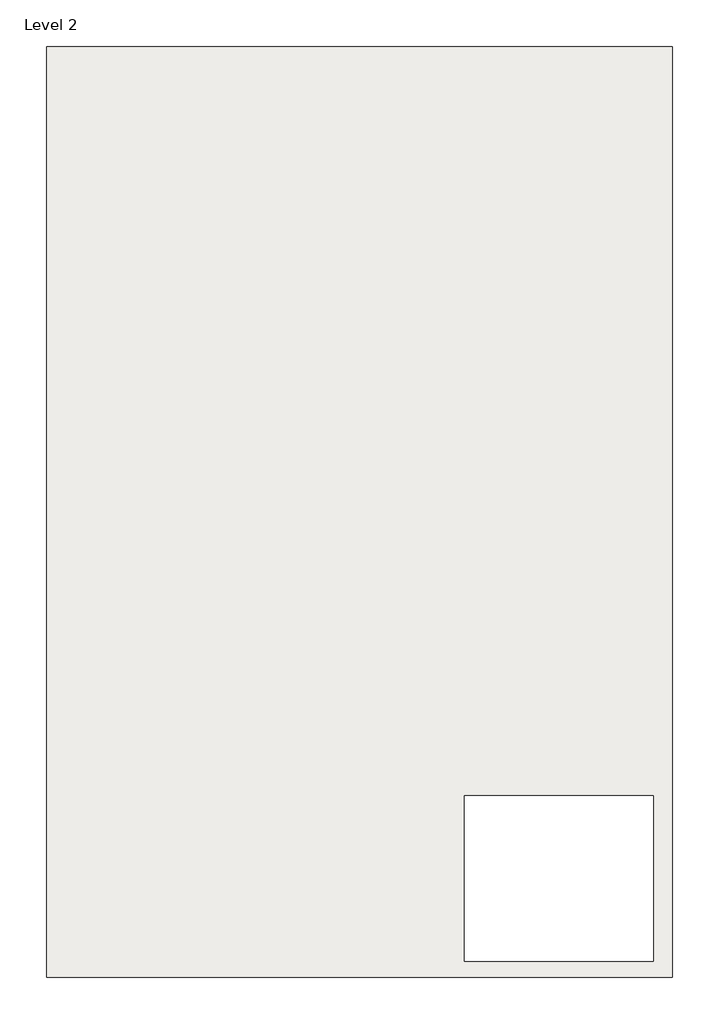
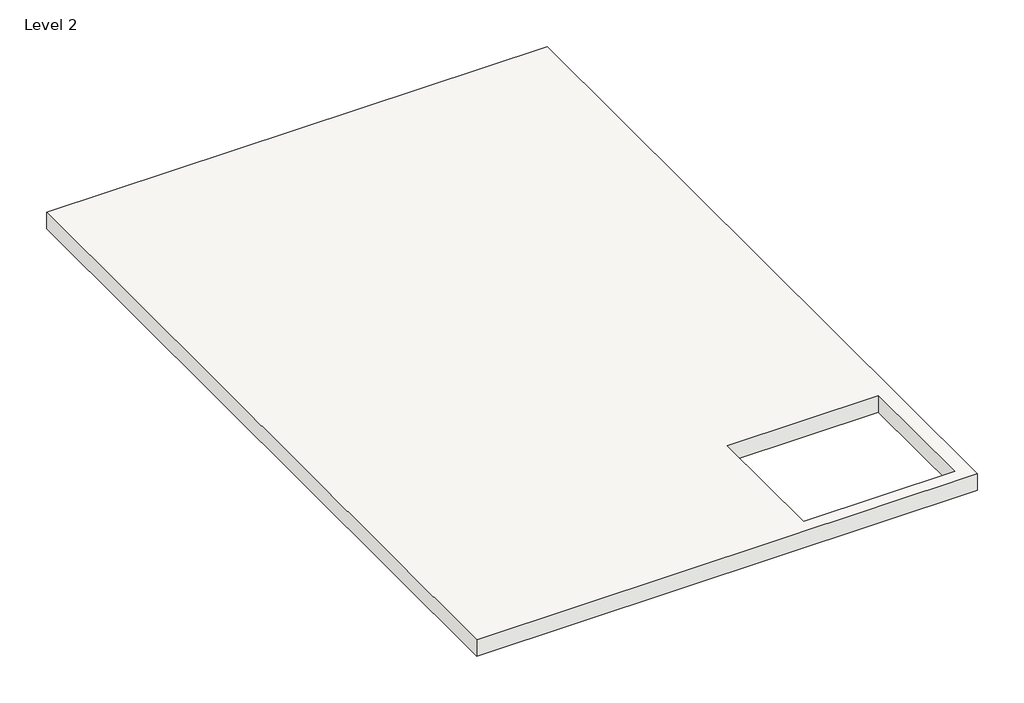
# One storey: 1 roof.
"""IFC4 building model written with IfcOpenShell, lengths in millimetres."""

from ifc_helpers import new_model, si_unit, frame, origin, place, context, project, spatial, polyline, outline, extrude, element, save

model = new_model("IFC4")

# Units and contexts
model_context = context("Model", 3, world=origin())
ifc_project = project(units=[si_unit("LENGTHUNIT", "METRE", prefix="MILLI")], contexts=[model_context])

# Site, building, storey
site = spatial("IfcSite", under=ifc_project)
building = spatial("IfcBuilding", under=site)
storey = spatial("IfcBuildingStorey", under=building, Name="Level 2", Elevation=3048.0)

# Roof
placement = place(None, origin())
element("IfcRoof", 1, ObjectType="Generic - 12\"", at=placement, inside=storey, context=model_context, shape_type="SweptSolid", body=[
    extrude(outline(polyline([(-12848.2505662, 13201.5645941), (-4085.2505662, 13201.5645941), (-4085.2505662, 171.3645941), (-12848.2505662, 171.3645941), (-12848.2505662, 13201.5645941)]), holes=[polyline([(-4351.9505662, 399.9645941), (-4351.9505662, 2711.3645941), (-6993.5505662, 2711.3645941), (-6993.5505662, 399.9645941), (-4351.9505662, 399.9645941)])]), frame((0.0, 0.0, 3048.0), z_axis=(0.0, 0.0, 1.0), x_axis=(1.0, 0.0, 0.0)), (0.0, 0.0, 1.0), 304.8),
])

save(model, "model.ifc")

# Revit data of these elements
# Type "Generic - 12\""
#   Assembly Code = "B1020"
#   Layers, outside or top first: 1' - 0" "Brick, Soldier Course" (function 1)
# Element 1 (IfcRoof, "Generic - 12\"")
#   built-in parameter 1001705 = 11 (stored number, unit not read)
#   built-in parameter 1001710 = 33615
#   Phase Created = New Construction
#   Materials on its faces: "Brick, Soldier Course"
# Materials
#   "Brick, Soldier Course": class "Masonry", colour RGB 170 98 104, transparency 0, Description = "Common brick soldier coursed", Cost = 0
